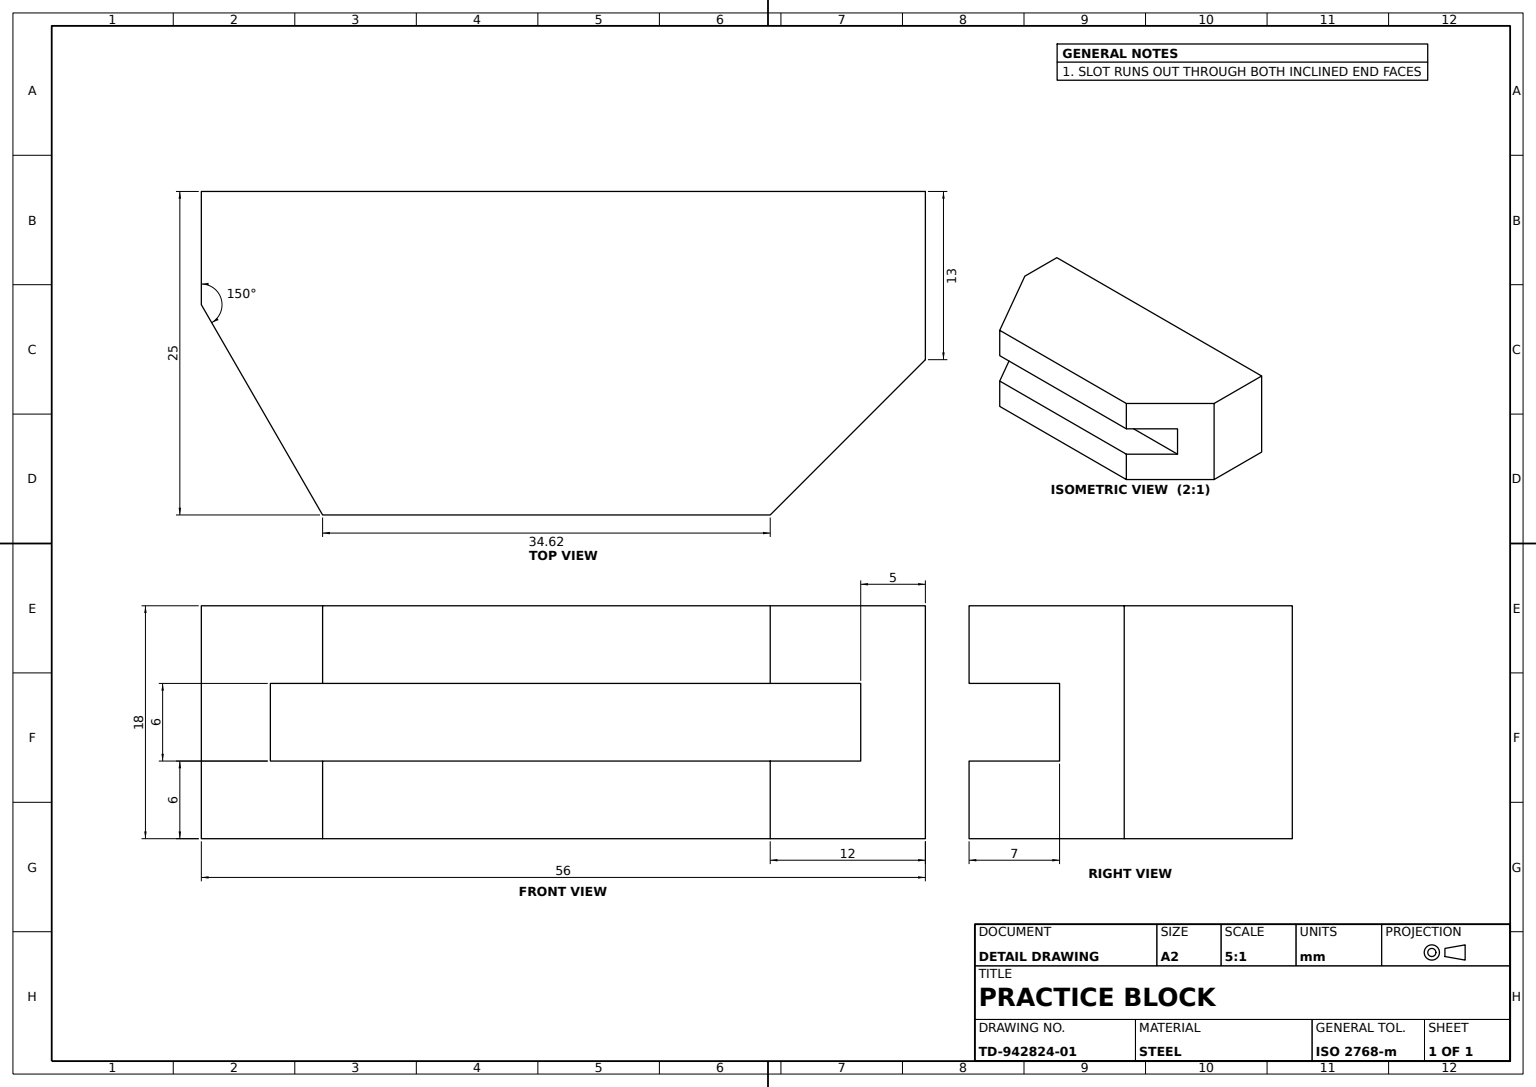
from build123d import *

# Parameters (mm, degrees)
BASE_PROFILE_SKETCH_W    = 56
BASE_PROFILE_SKETCH_H    = 18
BASE_BLOCK_DEPTH         = 25
ANGLED_CORNER_CUTS_DEPTH = 42.629316593
SLOT_SKETCH_W            = 47
SLOT_SKETCH_H            = 6
SLOT_47X6_DEPTH          = 7


with BuildPart() as part:
    # Base Profile Sketch → Base Block (new body)
    with BuildSketch(Plane.XY):
        Rectangle(BASE_PROFILE_SKETCH_W, BASE_PROFILE_SKETCH_H)
    extrude(amount=BASE_BLOCK_DEPTH)

    # Corner Cut Sketch → Angled Corner Cuts (cut, through all)
    with BuildSketch(Plane.XZ.offset(9)):
        Polygon((28, 13), (16, 25), (28, 25), align=None)
        Polygon((-28, 13), (-28, 8.753100352), (-18.619848115, 25), (-28, 25), align=None)
    extrude(amount=-ANGLED_CORNER_CUTS_DEPTH, mode=Mode.SUBTRACT)

    # Slot Sketch → Slot 47x6 (cut)
    with BuildSketch(Plane.XY.offset(25)):
        Rectangle(SLOT_SKETCH_W, SLOT_SKETCH_H)
    extrude(amount=-SLOT_47X6_DEPTH, mode=Mode.SUBTRACT)


solid = part.part
